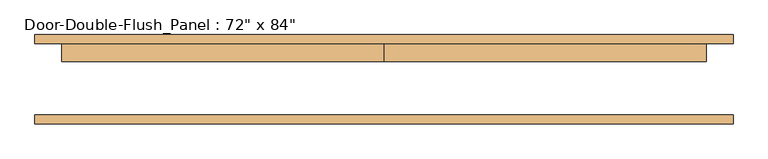
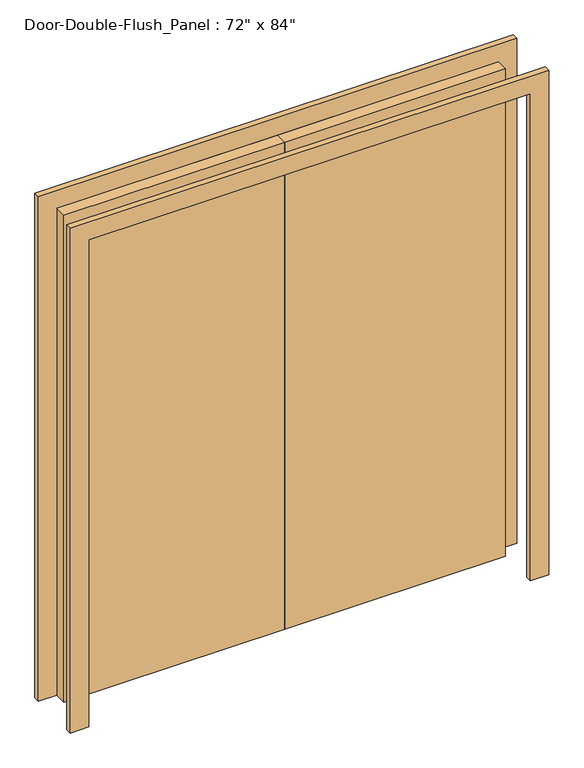
"""IFC4 building model written with IfcOpenShell, lengths in millimetres: door geometry."""

from ifc_helpers import new_model, si_unit, frame, origin, origin_with_axes, place, context, project, spatial, polyline, outline, extrude, source, transform, mapped, element, save


def door_0b985982(model_context):
    return source(origin(), model_context, "Body", "SweptSolid", [
        extrude(outline(polyline([(2133.6, -914.4), (2133.6, 914.4), (0.0, 914.4), (0.0, 990.6), (2209.8, 990.6), (2209.8, -990.6), (0.0, -990.6), (0.0, -914.4), (2133.6, -914.4)])), frame((0.0, -127.0, 0.0), z_axis=(0.0, 1.0, 0.0), x_axis=(0.0, 0.0, 1.0)), (0.0, 0.0, 1.0), 25.4),
        extrude(outline(polyline([(2133.6, -914.4), (2133.6, 914.4), (0.0, 914.4), (0.0, 990.6), (2209.8, 990.6), (2209.8, -990.6), (0.0, -990.6), (0.0, -914.4), (2133.6, -914.4)])), frame((0.0, 101.6, 0.0), z_axis=(0.0, 1.0, 0.0), x_axis=(0.0, 0.0, 1.0)), (0.0, 0.0, 1.0), 25.4),
        extrude(outline(polyline([(0.0, 101.6), (914.4, 101.6), (914.4, 50.8), (0.0, 50.8), (0.0, 101.6)])), origin_with_axes(), (0.0, 0.0, 1.0), 2133.6),
        extrude(outline(polyline([(-914.4, 101.6), (0.0, 101.6), (0.0, 50.8), (-914.4, 50.8), (-914.4, 101.6)])), origin_with_axes(), (0.0, 0.0, 1.0), 2133.6),
    ])


if __name__ == "__main__":
    model = new_model("IFC4")
    model_context = context("Model", 3, world=origin())
    ifc_project = project(units=[si_unit("LENGTHUNIT", "METRE", prefix="MILLI")], contexts=[model_context])
    site = spatial("IfcSite", under=ifc_project)
    building = spatial("IfcBuilding", under=site)
    placement = place(None, origin())
    door_shape = door_0b985982(model_context)
    element("IfcDoor", 1, ObjectType="Door-Double-Flush_Panel : 72\" x 84\"", at=placement, inside=building, context=model_context, shape_type="MappedRepresentation", body=[
        mapped(door_shape, transform((0.0, 0.0, 0.0), x_axis=(1.0, 0.0, 0.0), y_axis=(0.0, 1.0, 0.0), z_axis=(0.0, 0.0, 1.0))),
    ])
    save(model, "model.ifc")

# Revit data of these elements
# Type "Door-Double-Flush_Panel : 72\" x 84\""
#   Type Mark = "9"
#   Construction Type Id = "DOOR"
#   Assembly Code = "C1020"
#   Analytic Construction = "Wooden"
#   Thickness = 0' - 2"
#   Thermal Resistance (R) = 2.5876 (h·ft²·°F)/BTU
#   Swing Angle [instance default] = 90.00°
#   Panel Width = 3' - 0"
#   Heat Transfer Coefficient (U) = 0.3865 BTU/(h·ft²·°F)
#   Height = 7' - 0"
#   Trim Projection Ext = 0' - 1"
#   Trim Projection Int = 0' - 1"
#   Trim Width = 0' - 3"
#   Width = 6' - 0"
#   Define Thermal Properties by = 1
#   Panel Material = Earth
#   Trim Material = Paint - Sienna
#   Visual Light Transmittance = 0
#   Solar Heat Gain Coefficient = 0
#   Function = (empty or 0)
#   Wall Closure = (empty or 0)
# Element 1 (IfcDoor, "Door-Double-Flush_Panel : 72\" x 84\"")
#   Materials on its faces: "Paint - Sienna", "Earth"
# Materials
#   "Earth": class "Generic", colour RGB 97 75 62, transparency 0, Description = "Soil", Cost = 0
#   "Paint - Sienna": colour RGB 118 70 51, transparency 0, Cost = 0
